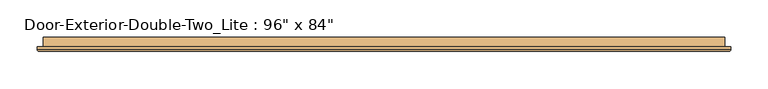
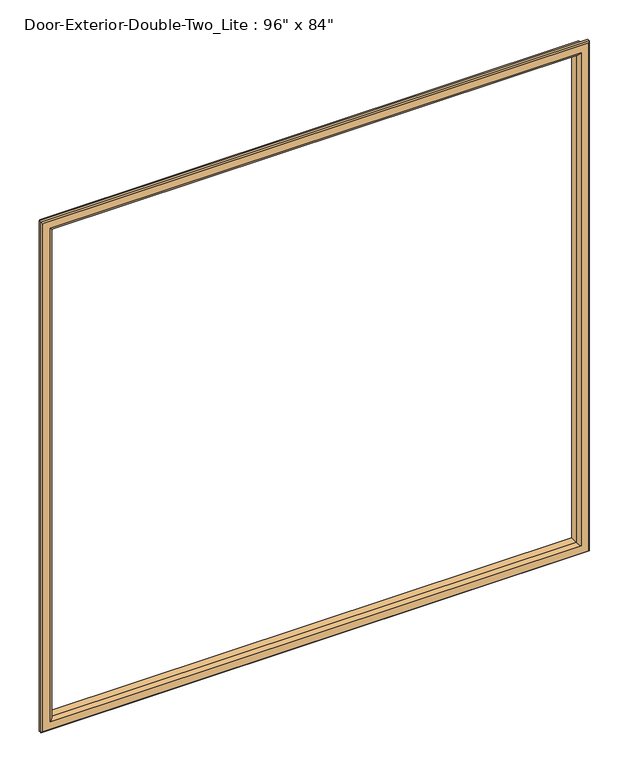
"""IFC4 building model written with IfcOpenShell, lengths in millimetres: door geometry."""

from ifc_helpers import new_model, si_unit, frame, origin, place, context, project, spatial, ellipse_curve, source, transform, mapped, element, save
from ifc_brep_helpers import plane_surface, cylinder_surface, advanced_brep


def door_1bf41894(model_context):
    return source(origin(), model_context, "Body", "AdvancedBrep", [
        advanced_brep(
        [(-1066.8, 50.8, 1117.6), (-1066.8, 38.1, 1117.6), (-1066.8, 38.1, 2016.125), (-1066.8, 50.8, 2016.125), (-1054.8, 37.1, 1129.6), (-1054.8, 50.8, 1129.6), (-1054.8, 50.8, 2004.125), (-1054.8, 37.1, 2004.125), (-1059.8, 32.1, 1124.6), (-1059.8, 32.1, 2009.125), (-1074.8, 34.1, 1109.6), (-1072.8, 32.1, 1111.6), (-1072.8, 32.1, 2022.125), (-1074.8, 34.1, 2024.125), (-1074.8, 38.1, 1109.6), (-1074.8, 38.1, 2024.125), (-152.4, 38.1, 2016.125), (-152.4, 50.8, 2016.125), (-164.4, 50.8, 2004.125), (-164.4, 37.1, 2004.125), (-159.4, 32.1, 2009.125), (-146.4, 32.1, 2022.125), (-144.4, 34.1, 2024.125), (-144.4, 38.1, 2024.125), (-152.4, 38.1, 1117.6), (-152.4, 50.8, 1117.6), (-164.4, 50.8, 1129.6), (-164.4, 37.1, 1129.6), (-159.4, 32.1, 1124.6), (-146.4, 32.1, 1111.6), (-144.4, 34.1, 1109.6), (-144.4, 38.1, 1109.6)],
        [
            (0, 1),
            (1, 2),
            (2, 3),
            (3, 0),
            (4, 5),
            (5, 6),
            (6, 7),
            (7, 4),
            (8, 4, ellipse_curve(frame((-1059.8, 37.1, 1124.6), z_axis=(-0.7071067811865475, 0.0, 0.7071067811865475), x_axis=(-0.7071067811865474, 0.0, -0.7071067811865476)), 7.0710678, 5.0)),
            (7, 9, ellipse_curve(frame((-1059.8, 37.1, 2009.125), z_axis=(-0.7071067811865475, 0.0, -0.7071067811865475), x_axis=(0.7071067811865474, 0.0, -0.7071067811865476)), 7.0710678, 5.0)),
            (9, 8),
            (10, 11, ellipse_curve(frame((-1072.8, 34.1, 1111.6), z_axis=(-0.7071067811865475, 0.0, 0.7071067811865475), x_axis=(-0.7071067811865474, 0.0, -0.7071067811865476)), 2.8284271, 2.0)),
            (11, 12),
            (12, 13, ellipse_curve(frame((-1072.8, 34.1, 2022.125), z_axis=(-0.7071067811865475, 0.0, -0.7071067811865475), x_axis=(0.7071067811865474, 0.0, -0.7071067811865476)), 2.8284271, 2.0)),
            (13, 10),
            (14, 10),
            (13, 15),
            (15, 14),
            (2, 16),
            (16, 17),
            (17, 3),
            (6, 18),
            (18, 19),
            (19, 7),
            (19, 20, ellipse_curve(frame((-159.4, 37.1, 2009.125), z_axis=(-0.7071067811865475, 0.0, 0.7071067811865475), x_axis=(-0.7071067811865476, 0.0, -0.7071067811865474)), 7.0710678, 5.0)),
            (20, 9),
            (12, 21),
            (21, 22, ellipse_curve(frame((-146.4, 34.1, 2022.125), z_axis=(-0.7071067811865475, 0.0, 0.7071067811865475), x_axis=(-0.7071067811865476, 0.0, -0.7071067811865474)), 2.8284271, 2.0)),
            (22, 13),
            (22, 23),
            (23, 15),
            (16, 24),
            (24, 25),
            (25, 17),
            (18, 26),
            (26, 27),
            (27, 19),
            (27, 28, ellipse_curve(frame((-159.4, 37.1, 1124.6), z_axis=(0.7071067811865475, 0.0, 0.7071067811865475), x_axis=(-0.7071067811865474, 0.0, 0.7071067811865476)), 7.0710678, 5.0)),
            (28, 20),
            (21, 29),
            (29, 30, ellipse_curve(frame((-146.4, 34.1, 1111.6), z_axis=(0.7071067811865475, 0.0, 0.7071067811865475), x_axis=(-0.7071067811865474, 0.0, 0.7071067811865476)), 2.8284271, 2.0)),
            (30, 22),
            (30, 31),
            (31, 23),
            (31, 14),
            (1, 24),
            (0, 25),
            (5, 26),
            (4, 27),
            (8, 28),
            (11, 29),
            (10, 30),
        ],
        [
            plane_surface(frame((-1066.8, 38.1, 1117.6), z_axis=(-1.0, 0.0, 0.0), x_axis=(0.0, 0.0, 1.0))),
            plane_surface(frame((-1054.8, 50.8, 1129.6), z_axis=(1.0, 0.0, 0.0), x_axis=(0.0, 0.0, 1.0))),
            cylinder_surface(frame((-1059.8, 37.1, 1117.6), z_axis=(0.0, 0.0, -1.0), x_axis=(-1.0, 0.0, 0.0)), 5.0),
            cylinder_surface(frame((-1072.8, 34.1, 1117.6), z_axis=(0.0, 0.0, -1.0), x_axis=(-1.0, 0.0, 0.0)), 2.0),
            plane_surface(frame((-1074.8, 34.1, 1109.6), z_axis=(-1.0, 0.0, 0.0), x_axis=(0.0, 0.0, 1.0))),
            plane_surface(frame((-1066.8, 38.1, 2016.125), z_axis=(0.0, 0.0, 1.0), x_axis=(1.0, 0.0, 0.0))),
            plane_surface(frame((-1054.8, 50.8, 2004.125), z_axis=(0.0, 0.0, -1.0), x_axis=(1.0, 0.0, 0.0))),
            cylinder_surface(frame((-1066.8, 37.1, 2009.125), z_axis=(-1.0, 0.0, 0.0), x_axis=(0.0, 0.0, 1.0)), 5.0),
            cylinder_surface(frame((-1066.8, 34.1, 2022.125), z_axis=(-1.0, 0.0, 0.0), x_axis=(0.0, 0.0, 1.0)), 2.0),
            plane_surface(frame((-1074.8, 34.1, 2024.125), z_axis=(0.0, 0.0, 1.0), x_axis=(1.0, 0.0, 0.0))),
            plane_surface(frame((-152.4, 38.1, 2016.125), z_axis=(1.0, 0.0, 0.0), x_axis=(0.0, 0.0, -1.0))),
            plane_surface(frame((-164.4, 50.8, 2004.125), z_axis=(-1.0, 0.0, 0.0), x_axis=(0.0, 0.0, -1.0))),
            cylinder_surface(frame((-159.4, 37.1, 2016.125), z_axis=(0.0, 0.0, 1.0), x_axis=(1.0, 0.0, 0.0)), 5.0),
            cylinder_surface(frame((-146.4, 34.1, 2016.125), z_axis=(0.0, 0.0, 1.0), x_axis=(1.0, 0.0, 0.0)), 2.0),
            plane_surface(frame((-144.4, 34.1, 2024.125), z_axis=(1.0, 0.0, 0.0), x_axis=(0.0, 0.0, -1.0))),
            plane_surface(frame((-144.4, 38.1, 1109.6), z_axis=(0.0, 1.0, 0.0), x_axis=(-1.0, 0.0, 0.0))),
            plane_surface(frame((-152.4, 38.1, 1117.6), z_axis=(0.0, 0.0, -1.0), x_axis=(-1.0, 0.0, 0.0))),
            plane_surface(frame((-152.4, 50.8, 1117.6), z_axis=(0.0, 1.0, 0.0), x_axis=(-1.0, 0.0, 0.0))),
            plane_surface(frame((-164.4, 50.8, 1129.6), z_axis=(0.0, 0.0, 1.0), x_axis=(-1.0, 0.0, 0.0))),
            cylinder_surface(frame((-152.4, 37.1, 1124.6), z_axis=(1.0, 0.0, 0.0), x_axis=(0.0, 0.0, -1.0)), 5.0),
            plane_surface(frame((-159.4, 32.1, 1124.6), z_axis=(0.0, -1.0, 0.0), x_axis=(-1.0, 0.0, 0.0))),
            cylinder_surface(frame((-152.4, 34.1, 1111.6), z_axis=(1.0, 0.0, 0.0), x_axis=(0.0, 0.0, -1.0)), 2.0),
            plane_surface(frame((-144.4, 34.1, 1109.6), z_axis=(0.0, 0.0, -1.0), x_axis=(-1.0, 0.0, 0.0))),
        ],
        [
            (0, [[1, 2, 3, 4]]),
            (1, [[5, 6, 7, 8]]),
            (2, [[9, -8, 10, 11]]),
            (3, [[12, 13, 14, 15]]),
            (4, [[16, -15, 17, 18]]),
            (5, [[-3, 19, 20, 21]]),
            (6, [[-7, 22, 23, 24]]),
            (7, [[-10, -24, 25, 26]]),
            (8, [[-14, 27, 28, 29]]),
            (9, [[-17, -29, 30, 31]]),
            (10, [[-20, 32, 33, 34]]),
            (11, [[-23, 35, 36, 37]]),
            (12, [[-25, -37, 38, 39]]),
            (13, [[-28, 40, 41, 42]]),
            (14, [[-30, -42, 43, 44]]),
            (15, [[-31, -44, 45, -18], [46, -32, -19, -2]]),
            (16, [[-33, -46, -1, 47]]),
            (17, [[-21, -34, -47, -4], [48, -35, -22, -6]]),
            (18, [[-36, -48, -5, 49]]),
            (19, [[-38, -49, -9, 50]]),
            (20, [[51, -40, -27, -13], [-26, -39, -50, -11]]),
            (21, [[-41, -51, -12, 52]]),
            (22, [[-43, -52, -16, -45]]),
        ],
    ),
    ])


if __name__ == "__main__":
    model = new_model("IFC4")
    model_context = context("Model", 3, world=origin())
    ifc_project = project(units=[si_unit("LENGTHUNIT", "METRE", prefix="MILLI")], contexts=[model_context])
    site = spatial("IfcSite", under=ifc_project)
    building = spatial("IfcBuilding", under=site)
    placement = place(None, origin())
    door_shape = door_1bf41894(model_context)
    element("IfcDoor", 1, ObjectType="Door-Exterior-Double-Two_Lite : 96\" x 84\"", at=placement, inside=building, context=model_context, shape_type="MappedRepresentation", body=[
        mapped(door_shape, transform((0.0, 0.0, 0.0), x_axis=(1.0, 0.0, 0.0), y_axis=(0.0, 1.0, 0.0), z_axis=(0.0, 0.0, 1.0))),
    ])
    save(model, "model.ifc")

# Revit data of these elements
# Type "Door-Exterior-Double-Two_Lite : 96\" x 84\""
#   Type Mark = "8"
#   Assembly Code = "B2030100"
#   Analytic Construction = "Metal frame, double glass door"
#   Top Rail = 0' - 4 5/8"
#   Threshold Length [instance default] = 8' - 4"
#   Threshold Offset [instance default] = 0' - 0 1/2"
#   Thickness = 0' - 1 3/4"
#   Thermal Resistance (R) = 1.3794 (h·ft²·°F)/BTU
#   Swing Angle [instance default] = 90.00°
#   Strike Height = 3' - 4"
#   Stiles = 0' - 6"
#   SinglePanelWidth = 4' - 0"
#   Rough Width [instance default] = 8' - 4"
#   Rough Height [instance default] = 7' - 4"
#   MFOpeningHeight [instance default] = 0' - 4"
#   MFOpeningWidth [instance default] = 0' - 4"
#   Lock Rail = 0' - 8"
#   Inset Calculate [instance default] = 0' - 4"
#   Masonry Inset [instance default] = 0' - 1"
#   Height = 7' - 0"
#   Width = 8' - 0"
#   Heat Transfer Coefficient (U) = 0.7250 BTU/(h·ft²·°F)
#   Glass Thickness = 0' - 0 3/4"
#   Masonry Frame Depth = 0' - 5 3/4"
#   Bottom Rail = 0' - 10"
#   Threshold [instance default] = yes
#   Masonry Frame [instance default] = yes
#   Wall Closure = 3
#   Function = 1
#   Dry Wall Frame [instance default] = no
#   Threshold Material = none
#   Panic Bar Material = Metal - Stainless Steel
#   Panel Material = Metal - Painted - Grey
#   Glass Stop Material = Metal - Painted - Grey
#   Frame Material = Metal - Painted - Grey
#   Exterior Pull Material = Metal - Stainless Steel
#   Visual Light Transmittance = 0
#   Solar Heat Gain Coefficient = 0
# Element 1 (IfcDoor, "Door-Exterior-Double-Two_Lite : 96\" x 84\"")
#   Materials on its faces: "Metal - Painted - Grey", "Metal - Stainless Steel", "Glass"
# Materials
#   "Metal - Stainless Steel": class "Metal", colour RGB 247 247 247, transparency 0
#   "Metal - Painted - Grey": class "Paint", colour RGB 104 104 104, transparency 0, Cost = 0
#   "Glass": class "Glass", colour RGB 0 128 192, transparency 0.75, Description = "Soda Lime Glass", Cost = 0
